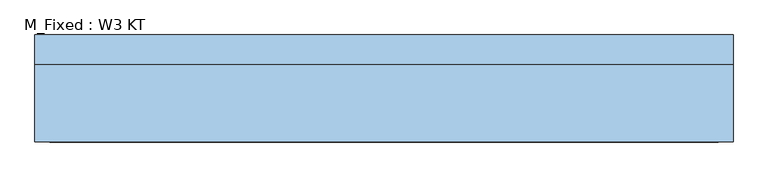
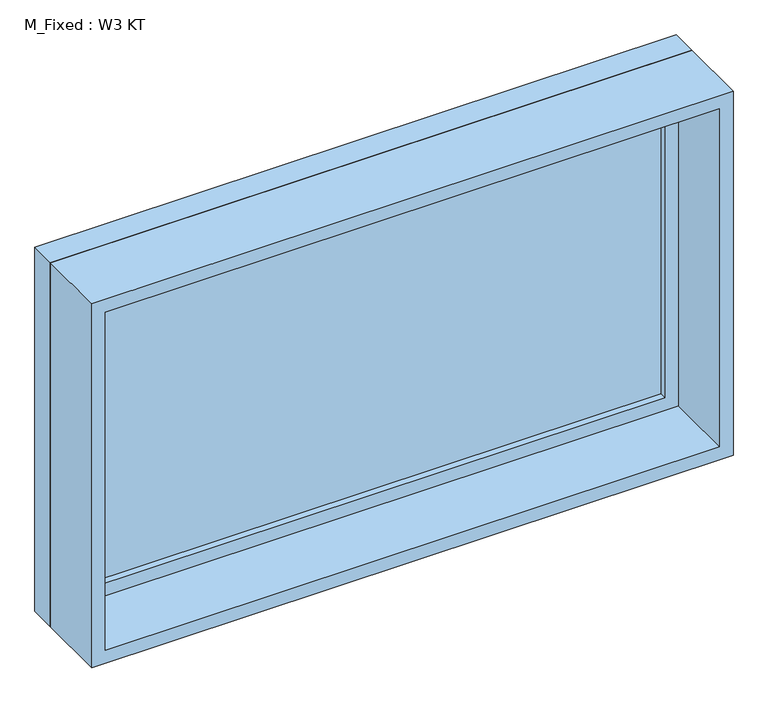
"""IFC4 building model written with IfcOpenShell, lengths in millimetres: window geometry, M_Fixed : W3 KT."""

from ifc_helpers import new_model, si_unit, frame, origin, place, context, project, spatial, polyline, outline, extrude, source, transform, mapped, element, save


def m_fixed_w3_kt_cae187e1(model_context):
    return source(origin(), model_context, "Body", "SweptSolid", [
        extrude(outline(polyline([(-687.0, 93.0), (687.0, 93.0), (687.0, 81.0), (-687.0, 81.0), (-687.0, 93.0)])), frame((0.0, 0.0, 1263.0), z_axis=(0.0, 0.0, 1.0), x_axis=(1.0, 0.0, 0.0)), (0.0, 0.0, 1.0), 774.0),
        extrude(outline(polyline([(2081.0, -731.0), (1219.0, -731.0), (1219.0, 731.0), (2081.0, 731.0), (2081.0, -731.0)]), holes=[polyline([(2037.0, -687.0), (2037.0, 687.0), (1263.0, 687.0), (1263.0, -687.0), (2037.0, -687.0)])]), frame((0.0, 65.0, 0.0), z_axis=(0.0, 1.0, 0.0), x_axis=(0.0, 0.0, 1.0)), (0.0, 0.0, 1.0), 44.0),
        extrude(outline(polyline([(2100.0, -750.0), (1200.0, -750.0), (1200.0, 750.0), (2100.0, 750.0), (2100.0, -750.0)]), holes=[polyline([(2081.0, -731.0), (2081.0, 731.0), (1219.0, 731.0), (1219.0, -731.0), (2081.0, -731.0)])]), frame((0.0, 65.0, 0.0), z_axis=(0.0, 1.0, 0.0), x_axis=(0.0, 0.0, 1.0)), (0.0, 0.0, 1.0), 63.0),
        extrude(outline(polyline([(2100.0, -750.0), (1200.0, -750.0), (1200.0, 750.0), (2100.0, 750.0), (2100.0, -750.0)]), holes=[polyline([(2068.0, -718.0), (2068.0, 718.0), (1232.0, 718.0), (1232.0, -718.0), (2068.0, -718.0)])]), frame((0.0, -102.0, 0.0), z_axis=(0.0, 1.0, 0.0), x_axis=(0.0, 0.0, 1.0)), (0.0, 0.0, 1.0), 167.0),
    ])


if __name__ == "__main__":
    model = new_model("IFC4")
    model_context = context("Model", 3, world=origin())
    ifc_project = project(units=[si_unit("LENGTHUNIT", "METRE", prefix="MILLI")], contexts=[model_context])
    site = spatial("IfcSite", under=ifc_project)
    building = spatial("IfcBuilding", under=site)
    placement = place(None, origin())
    m_fixed_w3_kt_shape = m_fixed_w3_kt_cae187e1(model_context)
    element("IfcWindow", 1, ObjectType="M_Fixed : W3 KT", at=placement, inside=building, context=model_context, shape_type="MappedRepresentation", body=[
        mapped(m_fixed_w3_kt_shape, transform((0.0, 0.0, 0.0), x_axis=(1.0, 0.0, 0.0), y_axis=(0.0, 1.0, 0.0), z_axis=(0.0, 0.0, 1.0))),
    ])
    save(model, "model.ifc")

# Revit data of these elements
# Type "M_Fixed : W3 KT"
#   Type Mark = "21"
#   Height = 900 mm
#   Default Sill Height = 1200 mm
#   Width = 1500 mm
#   Window Inset = 19 mm
#   Frame Exterior Material = Iron, Ductile
#   Frame Interior Material = Iron, Ductile
#   Glass Pane Material = Glass
#   Sash = Iron, Ductile
#   Wall Closure = (empty or 0)
# Element 1 (IfcWindow, "M_Fixed : W3 KT")
#   Materials on its faces: "Iron, Ductile", "Glass"
# Materials
#   "Iron, Ductile": class "Metal", colour RGB 90 97 102, transparency 0, Description = "Ductile cast iron", Cost = 0
#   "Glass": class "Glass", colour RGB 218 227 224, transparency 0.85, Description = "Soda Lime Glass", Cost = 0
